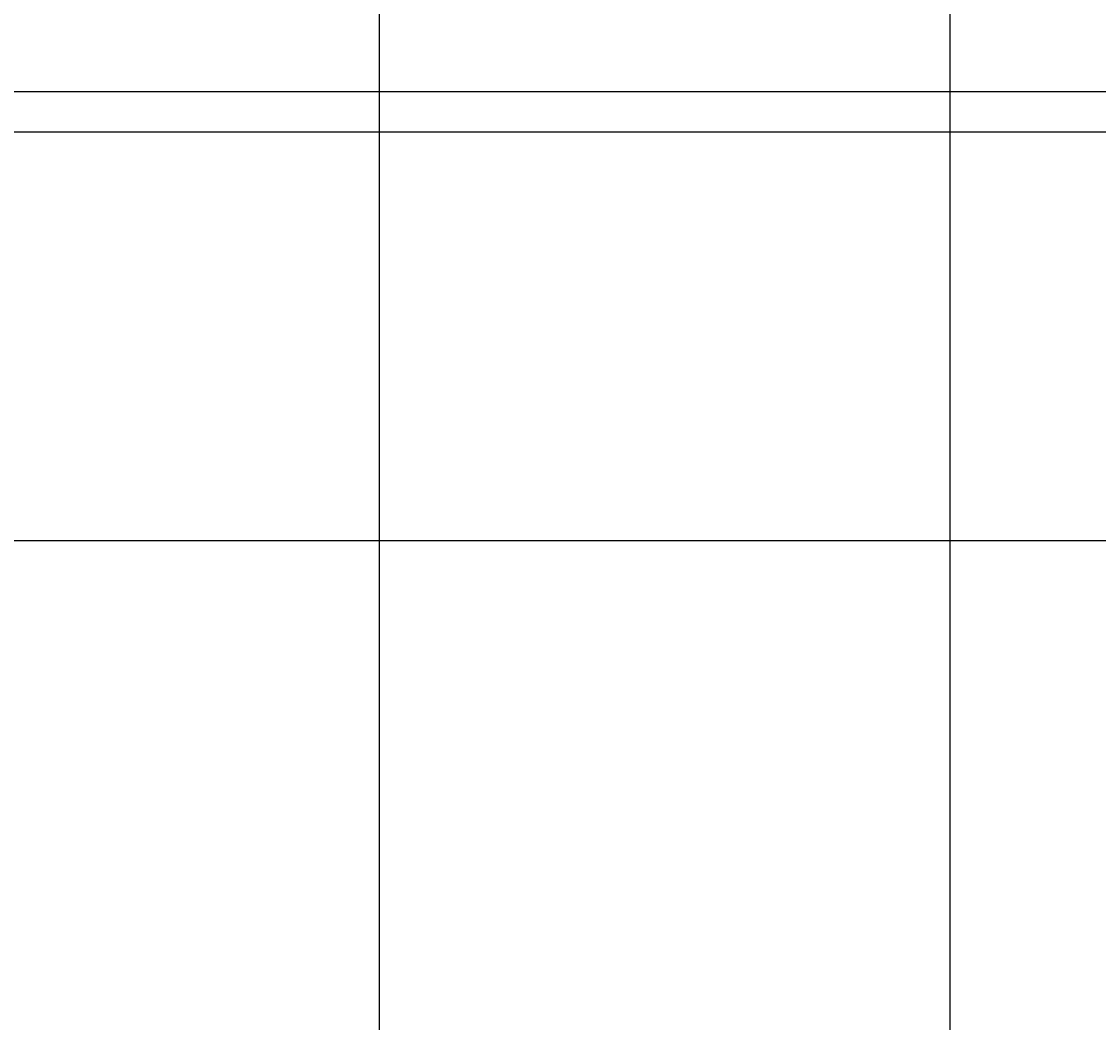
# Model space of a CAD drawing. Units: inches. Extents: x 35362 to 73946, y 43607 to 67532.
# Tile 121 of 134: x 50905 to 51049, y 49195 to 49329. Entities that reach past the tile are written whole.
import ezdxf

# ---------------------------------------------------------------- set-up
doc = ezdxf.new("R2010")
doc.units = ezdxf.units.IN
doc.header["$MEASUREMENT"] = 0
doc.layers.add('A-ANNO-DIMS', color=2, linetype='Continuous', lineweight=18)
doc.styles.get("Standard").update_dxf_attribs({"font": 'arial.ttf'})
doc.dimstyles.get("Standard").update_dxf_attribs({"dimtxt": 0.18, "dimasz": 0.18, "dimexe": 0.18, "dimexo": 0.0625, "dimgap": 0.09, "dimtad": 0, "dimtih": 1, "dimtoh": 1, "dimdec": 4, "dimzin": 0, "dimdsep": 46, "dimtxsty": 'Standard', "dimcen": 0.09, "dimadec": 0, "dimazin": 0, "dimtfac": 1, "dimtdec": 4, "dimtofl": 0, "dimtmove": 0, "dimatfit": 3, "dimfxl": 1, "dimtolj": 1, "dimtzin": 0, "dimarcsym": 0})

# ---------------------------------------------------------------- blocks, each defined once
blk = doc.blocks.new('*D11')
at = {"layer": 'A-ANNO-DIMS', "color": 0, "lineweight": -2, "transparency": 16777216}
for p, q in [((47978.66, 56028.77), (47978.66, 43606.68)), ((53109.76, 56028.77), (53109.76, 43606.68)), ((47978.84, 43606.86), (50543.87, 43606.86)), ((53109.58, 43606.86), (50544.55, 43606.86))]:
    blk.add_line(p, q, dxfattribs=at)
at = {"layer": 'A-ANNO-DIMS', "color": 0, "transparency": 16777216}
for points in [[(47978.84, 43606.89), (47978.84, 43606.83), (47978.66, 43606.86)], [(53109.58, 43606.89), (53109.58, 43606.83), (53109.76, 43606.86)]]:
    blk.add_solid(points, dxfattribs=at)
at = {"layer": 'Defpoints', "color": 0, "transparency": 16777216}
for p in [(47978.66, 56028.84), (53109.76, 56028.84), (53109.76, 43606.86)]:
    blk.add_point(p, dxfattribs=at)
at = {"layer": 'A-ANNO-DIMS', "color": 0, "transparency": 16777216, "insert": (50544.21, 43606.86), "char_height": 0.18, "attachment_point": 5}
blk.add_mtext('\\A1;5131', dxfattribs=at)
blk = doc.blocks.new('*D13')
at = {"layer": 'A-ANNO-DIMS', "color": 0, "lineweight": -2, "transparency": 16777216}
for p, q in [((48373.49, 51694.02), (48373.49, 43606.68)), ((51029.04, 51694.02), (51029.04, 43606.68)), ((48373.67, 43606.86), (49700.8, 43606.86)), ((51028.86, 43606.86), (49701.73, 43606.86))]:
    blk.add_line(p, q, dxfattribs=at)
at = {"layer": 'A-ANNO-DIMS', "color": 0, "transparency": 16777216}
for points in [[(48373.67, 43606.89), (48373.67, 43606.83), (48373.49, 43606.86)], [(51028.86, 43606.89), (51028.86, 43606.83), (51029.04, 43606.86)]]:
    blk.add_solid(points, dxfattribs=at)
at = {"layer": 'Defpoints', "color": 0, "transparency": 16777216}
for p in [(48373.49, 51694.09), (51029.04, 51694.09), (51029.04, 43606.86)]:
    blk.add_point(p, dxfattribs=at)
at = {"layer": 'A-ANNO-DIMS', "color": 0, "transparency": 16777216, "insert": (49701.27, 43606.86), "char_height": 0.18, "attachment_point": 5}
blk.add_mtext('\\A1;2655.6', dxfattribs=at)
blk = doc.blocks.new('*D17')
at = {"layer": 'A-ANNO-DIMS', "color": 0, "lineweight": -2, "transparency": 16777216}
for p, q in [((49923.31, 61293.22), (49923.31, 43606.68)), ((51913.93, 61293.22), (51913.93, 43606.68)), ((49923.49, 43606.86), (50918.16, 43606.86)), ((51913.75, 43606.86), (50919.07, 43606.86))]:
    blk.add_line(p, q, dxfattribs=at)
at = {"layer": 'A-ANNO-DIMS', "color": 0, "transparency": 16777216}
for points in [[(49923.49, 43606.89), (49923.49, 43606.83), (49923.31, 43606.86)], [(51913.75, 43606.89), (51913.75, 43606.83), (51913.93, 43606.86)]]:
    blk.add_solid(points, dxfattribs=at)
at = {"layer": 'Defpoints', "color": 0, "transparency": 16777216}
for p in [(49923.31, 61293.29), (51913.93, 61293.29), (51913.93, 43606.86)]:
    blk.add_point(p, dxfattribs=at)
at = {"layer": 'A-ANNO-DIMS', "color": 0, "transparency": 16777216, "insert": (50918.62, 43606.86), "char_height": 0.18, "attachment_point": 5}
blk.add_mtext('\\A1;1990.6', dxfattribs=at)
blk = doc.blocks.new('*D40')
at = {"layer": 'A-ANNO-DIMS', "color": 0, "lineweight": -2, "transparency": 16777216}
for p, q in [((56873.54, 53351.53), (35361.77, 53351.53)), ((35361.95, 53351.35), (35361.95, 51333.28)), ((35361.95, 49314.85), (35361.95, 51332.92)), ((51806.45, 49314.67), (35361.77, 49314.67))]:
    blk.add_line(p, q, dxfattribs=at)
at = {"layer": 'A-ANNO-DIMS', "color": 0, "transparency": 16777216}
for points in [[(35361.92, 53351.35), (35361.98, 53351.35), (35361.95, 53351.53)], [(35361.92, 49314.85), (35361.98, 49314.85), (35361.95, 49314.67)]]:
    blk.add_solid(points, dxfattribs=at)
at = {"layer": 'Defpoints', "color": 0, "transparency": 16777216}
for p in [(35361.95, 53351.53), (56873.6, 53351.53), (51806.52, 49314.67)]:
    blk.add_point(p, dxfattribs=at)
at = {"layer": 'A-ANNO-DIMS', "color": 0, "transparency": 16777216, "insert": (35361.95, 51333.1), "char_height": 0.18, "attachment_point": 5}
blk.add_mtext('\\A1;4036.9', dxfattribs=at)
blk = doc.blocks.new('*D67')
at = {"layer": 'A-ANNO-DIMS', "color": 0, "lineweight": -2, "transparency": 16777216}
for p, q in [((56873.54, 53351.53), (35361.77, 53351.53)), ((35361.95, 53351.35), (35361.95, 49400.89)), ((35361.95, 45450.07), (35361.95, 49400.53)), ((53793.58, 45449.89), (35361.77, 45449.89))]:
    blk.add_line(p, q, dxfattribs=at)
at = {"layer": 'A-ANNO-DIMS', "color": 0, "transparency": 16777216}
for points in [[(35361.92, 53351.35), (35361.98, 53351.35), (35361.95, 53351.53)], [(35361.92, 45450.07), (35361.98, 45450.07), (35361.95, 45449.89)]]:
    blk.add_solid(points, dxfattribs=at)
at = {"layer": 'Defpoints', "color": 0, "transparency": 16777216}
for p in [(35361.95, 53351.53), (56873.6, 53351.53), (53793.64, 45449.89)]:
    blk.add_point(p, dxfattribs=at)
at = {"layer": 'A-ANNO-DIMS', "color": 0, "transparency": 16777216, "insert": (35361.95, 49400.71), "char_height": 0.18, "attachment_point": 5}
blk.add_mtext('\\A1;7901.6', dxfattribs=at)
blk = doc.blocks.new('*D84')
at = {"layer": 'A-ANNO-DIMS', "color": 0, "lineweight": -2, "transparency": 16777216}
for p, q in [((55540.23, 49259.94), (35361.77, 49259.94)), ((35361.95, 49259.76), (35361.95, 49115.14)), ((35361.95, 48970.16), (35361.95, 49114.78)), ((55540.23, 48969.98), (35361.77, 48969.98))]:
    blk.add_line(p, q, dxfattribs=at)
at = {"layer": 'A-ANNO-DIMS', "color": 0, "transparency": 16777216}
for points in [[(35361.92, 49259.76), (35361.98, 49259.76), (35361.95, 49259.94)], [(35361.92, 48970.16), (35361.98, 48970.16), (35361.95, 48969.98)]]:
    blk.add_solid(points, dxfattribs=at)
at = {"layer": 'Defpoints', "color": 0, "transparency": 16777216}
for p in [(35361.95, 49259.94), (55540.3, 49259.94), (55540.3, 48969.98)]:
    blk.add_point(p, dxfattribs=at)
at = {"layer": 'A-ANNO-DIMS', "color": 0, "transparency": 16777216, "insert": (35361.95, 49114.96), "char_height": 0.18, "attachment_point": 5}
blk.add_mtext('\\A1;289.96', dxfattribs=at)
blk = doc.blocks.new('*D85')
at = {"layer": 'A-ANNO-DIMS', "color": 0, "lineweight": -2, "transparency": 16777216}
for p, q in [((50952.66, 49098.43), (50952.66, 67531.69)), ((51285.59, 49320.14), (51285.59, 67531.69)), ((50952.84, 67531.51), (51118.73, 67531.51)), ((51285.41, 67531.51), (51119.52, 67531.51))]:
    blk.add_line(p, q, dxfattribs=at)
at = {"layer": 'A-ANNO-DIMS', "color": 0, "transparency": 16777216}
for points in [[(50952.84, 67531.54), (50952.84, 67531.48), (50952.66, 67531.51)], [(51285.41, 67531.54), (51285.41, 67531.48), (51285.59, 67531.51)]]:
    blk.add_solid(points, dxfattribs=at)
at = {"layer": 'Defpoints', "color": 0, "transparency": 16777216}
for p in [(51285.59, 67531.51), (51285.59, 49320.08), (50952.66, 49098.37)]:
    blk.add_point(p, dxfattribs=at)
at = {"layer": 'A-ANNO-DIMS', "color": 0, "transparency": 16777216, "insert": (51119.13, 67531.51), "char_height": 0.18, "attachment_point": 5}
blk.add_mtext('\\A1;332.9', dxfattribs=at)
blk = doc.blocks.new('*D86')
at = {"layer": 'A-ANNO-DIMS', "color": 0, "lineweight": -2, "transparency": 16777216}
for p, q in [((51285.53, 49320.08), (35361.77, 49320.08)), ((35361.95, 49319.9), (35361.95, 49120.26)), ((35361.95, 48920.26), (35361.95, 49119.9)), ((51285.53, 48920.08), (35361.77, 48920.08))]:
    blk.add_line(p, q, dxfattribs=at)
at = {"layer": 'A-ANNO-DIMS', "color": 0, "transparency": 16777216}
for points in [[(35361.92, 49319.9), (35361.98, 49319.9), (35361.95, 49320.08)], [(35361.92, 48920.26), (35361.98, 48920.26), (35361.95, 48920.08)]]:
    blk.add_solid(points, dxfattribs=at)
at = {"layer": 'Defpoints', "color": 0, "transparency": 16777216}
for p in [(35361.95, 49320.08), (51285.59, 49320.08), (51285.59, 48920.08)]:
    blk.add_point(p, dxfattribs=at)
at = {"layer": 'A-ANNO-DIMS', "color": 0, "transparency": 16777216, "insert": (35361.95, 49120.08), "char_height": 0.18, "attachment_point": 5}
blk.add_mtext('\\A1;400.0', dxfattribs=at)
blk = doc.blocks.new('*D107')
at = {"layer": 'A-ANNO-DIMS', "color": 0, "lineweight": -2, "transparency": 16777216}
for p, q in [((50139.56, 59850.01), (50139.56, 43606.68)), ((51320.81, 59850.01), (51320.81, 43606.68)), ((50139.74, 43606.86), (50729.73, 43606.86)), ((51320.63, 43606.86), (50730.64, 43606.86))]:
    blk.add_line(p, q, dxfattribs=at)
at = {"layer": 'A-ANNO-DIMS', "color": 0, "transparency": 16777216}
for points in [[(50139.74, 43606.89), (50139.74, 43606.83), (50139.56, 43606.86)], [(51320.63, 43606.89), (51320.63, 43606.83), (51320.81, 43606.86)]]:
    blk.add_solid(points, dxfattribs=at)
at = {"layer": 'Defpoints', "color": 0, "transparency": 16777216}
for p in [(50139.56, 59850.08), (51320.81, 59850.08), (51320.81, 43606.86)]:
    blk.add_point(p, dxfattribs=at)
at = {"layer": 'A-ANNO-DIMS', "color": 0, "transparency": 16777216, "insert": (50730.19, 43606.86), "char_height": 0.18, "attachment_point": 5}
blk.add_mtext('\\A1;1181.3', dxfattribs=at)

msp = doc.modelspace()

# ---------------------------------------------------------------- dimensions: what is measured, and where the dimension line sits
at = {"layer": 'A-ANNO-DIMS'}
for base, p1, p2, override, picture, middle in [((51285.595, 67531.512), (50952.662, 49098.368), (51285.595, 49320.079), {"dimdec": 1, "dimlfac": 1, "dimrnd": 0, "dimzin": 0, "dimdsep": 46, "dimlunit": 2}, '*D85', (51119.128, 67531.512)), ((51913.931, 43606.859), (49923.307, 61293.286), (51913.931, 61293.286), {"dimdec": 1, "dimlfac": 1, "dimrnd": 0, "dimzin": 0, "dimdsep": 46, "dimlunit": 2}, '*D17', (50918.619, 43606.859)), ((51320.8133, 43606.859), (50139.5627, 59850.0769), (51320.8133, 59850.0769), {"dimdec": 1, "dimlfac": 1, "dimrnd": 0, "dimzin": 0, "dimdsep": 46, "dimlunit": 2}, '*D107', (50730.188, 43606.859)), ((53109.76, 43606.859), (47978.665, 56028.836), (53109.76, 56028.836), {"dimdec": 0, "dimlfac": 1, "dimrnd": 0, "dimzin": 0, "dimdsep": 46, "dimlunit": 2}, '*D11', (50544.212, 43606.859)), ((51029.043, 43606.859), (48373.492, 51694.087), (51029.043, 51694.087), {"dimdec": 1, "dimlfac": 1, "dimrnd": 0, "dimzin": 0, "dimdsep": 46, "dimlunit": 2}, '*D13', (49701.267, 43606.859))]:
    dim = msp.add_linear_dim(base=base, p1=p1, p2=p2, dimstyle='Standard', override=override, dxfattribs=at)
    dim.commit()
    dim.dimension.update_dxf_attribs({"geometry": picture, "text_midpoint": middle})
for base, p1, p2, override, picture, middle in [((35361.949, 53351.529), (51806.517, 49314.669), (56873.602, 53351.529), {"dimdec": 1, "dimlfac": 1, "dimrnd": 0, "dimzin": 0, "dimdsep": 46, "dimlunit": 2}, '*D40', (35361.949, 51333.099)), ((35361.949, 53351.529), (53793.638, 45449.894), (56873.602, 53351.529), {"dimdec": 1, "dimlfac": 1, "dimrnd": 0, "dimzin": 0, "dimdsep": 46, "dimlunit": 2}, '*D67', (35361.949, 49400.712)), ((35361.949, 49320.079), (51285.595, 48920.079), (51285.595, 49320.079), {"dimdec": 1, "dimlfac": 1, "dimrnd": 0, "dimzin": 0, "dimdsep": 46, "dimlunit": 2}, '*D86', (35361.949, 49120.079)), ((35361.9491, 49259.9353), (55540.2972, 48969.9796), (55540.2972, 49259.9353), {"dimdec": 2, "dimlfac": 1, "dimrnd": 0, "dimzin": 0, "dimdsep": 46, "dimlunit": 2}, '*D84', (35361.9491, 49114.9575))]:
    dim = msp.add_linear_dim(base=base, p1=p1, p2=p2, angle=90, dimstyle='Standard', override=override, dxfattribs=at)
    dim.commit()
    dim.dimension.update_dxf_attribs({"geometry": picture, "text_midpoint": middle})

doc.saveas('drawing.dxf')
